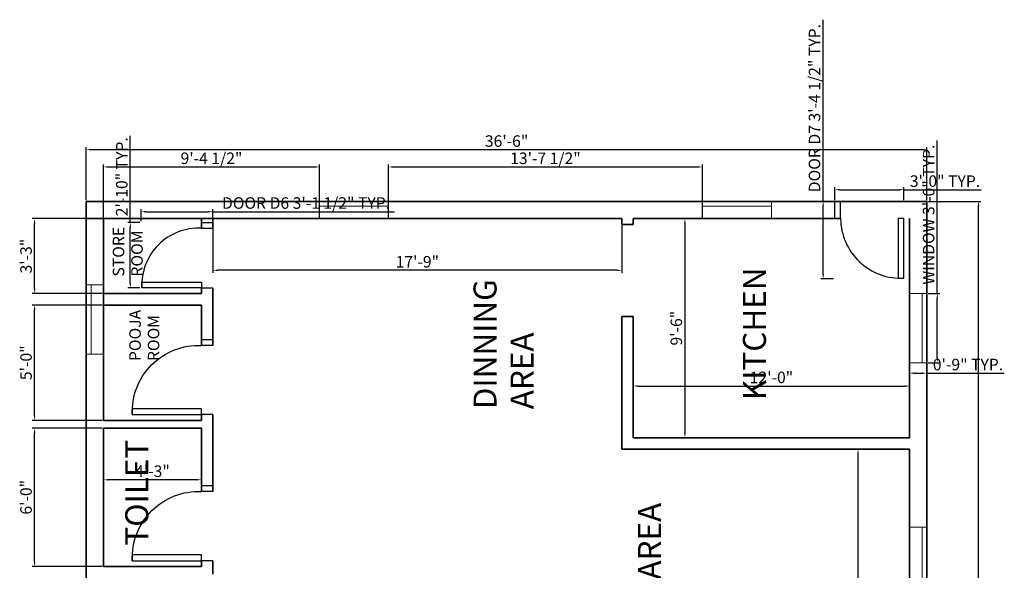
# Model space of a CAD drawing. Units: inches. Extents: x 2641 to 3210, y 2696 to 4064.
# Tile 4 of 4: x 2645 to 3158, y 3777 to 4064. Entities that reach past the tile are written whole.
import ezdxf

# ---------------------------------------------------------------- set-up
doc = ezdxf.new("R2010")
doc.units = ezdxf.units.IN
for name, color, linetype, lineweight in [('A-ANNO-DIMS', 2, 'Continuous', 18), ('A-AREA-IDEN', 7, 'Continuous', 18), ('A-DOOR', 3, 'Continuous', 25), ('A-GLAZ', 4, 'Continuous', 18), ('A-WALL', 7, 'Continuous', 35)]:
    doc.layers.add(name, color=color, linetype=linetype, lineweight=lineweight)
doc.styles.get("Standard").update_dxf_attribs({"font": 'arial.ttf'})
doc.dimstyles.new('ISO-25', dxfattribs={"dimtxt": 6, "dimasz": 2.5, "dimexe": 1.25, "dimexo": 0.625, "dimtad": 1, "dimdec": 1, "dimlunit": 3, "dimtxsty": 'Standard', "dimcen": 2.5, "dimadec": 0, "dimazin": 0, "dimtfac": 1, "dimtdec": 1, "dimtmove": 0, "dimatfit": 3, "dimfxl": 1, "dimarcsym": 0})

# ---------------------------------------------------------------- blocks, each defined once
blk = doc.blocks.new('DOOR-36-INT')
for p, q in [((0, 42.03), (0, 36.03)), ((36, 42.03), (36, 36.03)), ((39, 42.03), (39, 36.03))]:
    blk.add_line(p, q)
blk.add_lwpolyline([(0, 36.03), (3, 36.03), (3, 0.03), (0, 0.03)], close=True)
blk.add_arc((1.5, 34.53), 34.53, 267.5104, 2.4896)
blk = doc.blocks.new('DOOR-31-INT')
for p, q in [((31.04, 34), (37.04, 34)), ((31.04, 31), (37.04, 31)), ((31.04, 0), (37.04, 0))]:
    blk.add_line(p, q)
blk.add_lwpolyline([(31.04, 0), (0.04, 0), (0.04, 3), (31.04, 3)], close=True)
blk.add_arc((29.54, 1.5), 29.54, 87.0892, 182.9108)
blk = doc.blocks.new('DOOR-31-EXT')
for p, q in [((0, 31.04), (0, 40.04)), ((3, 31.04), (3, 40.04))]:
    blk.add_line(p, q)
blk.add_lwpolyline([(36, 31.04), (33, 31.04), (33, 0.04), (36, 0.04)], close=True)
blk.add_arc((34.5, 31.5), 31.5, 180.8507, 272.7291)
blk = doc.blocks.new('WIN-36x9')
blk.add_line((6.5, 36), (6.5, 0))
blk.add_lwpolyline([(9, 36), (0, 36), (0, 0), (9, 0)], close=True)
blk = doc.blocks.new('*D31')
at = {"layer": 'A-ANNO-DIMS', "color": 0, "lineweight": -2, "transparency": 16777216}
for p, q in [((3123.03, 3921.39), (3123.03, 4001.07)), ((3118.25, 3921.39), (3124.28, 3921.39)), ((3123.03, 3887.89), (3123.03, 3918.89)), ((3118.25, 3885.39), (3124.28, 3885.39))]:
    blk.add_line(p, q, dxfattribs=at)
at = {"layer": 'A-ANNO-DIMS', "color": 0, "transparency": 16777216}
for points in [[(3122.61, 3918.89), (3123.44, 3918.89), (3123.03, 3921.39)], [(3122.61, 3887.89), (3123.44, 3887.89), (3123.03, 3885.39)]]:
    blk.add_solid(points, dxfattribs=at)
at = {"layer": 'Defpoints', "color": 0, "transparency": 16777216}
for p in [(3117.63, 3921.39), (3123.03, 3921.39), (3117.63, 3885.39)]:
    blk.add_point(p, dxfattribs=at)
at = {"layer": 'A-ANNO-DIMS', "color": 0, "transparency": 16777216, "insert": (3119.29, 3962.48), "char_height": 6, "attachment_point": 5, "rotation": 90}
blk.add_mtext('WINDOW 3\'-0" TYP.', dxfattribs=at)
blk = doc.blocks.new('*D32')
at = {"layer": 'A-ANNO-DIMS', "color": 0, "lineweight": -2, "transparency": 16777216}
for p, q in [((3108.63, 3884.77), (3108.63, 3878.74)), ((3117.63, 3884.77), (3117.63, 3878.74)), ((3111.13, 3879.99), (3115.13, 3879.99)), ((3117.63, 3879.99), (3157.95, 3879.99))]:
    blk.add_line(p, q, dxfattribs=at)
at = {"layer": 'A-ANNO-DIMS', "color": 0, "transparency": 16777216}
for points in [[(3111.13, 3880.41), (3111.13, 3879.57), (3108.63, 3879.99)], [(3115.13, 3880.41), (3115.13, 3879.57), (3117.63, 3879.99)]]:
    blk.add_solid(points, dxfattribs=at)
at = {"layer": 'Defpoints', "color": 0, "transparency": 16777216}
for p in [(3108.63, 3885.39), (3117.63, 3885.39), (3117.63, 3879.99)]:
    blk.add_point(p, dxfattribs=at)
at = {"layer": 'A-ANNO-DIMS', "color": 0, "transparency": 16777216, "insert": (3139.04, 3883.68), "char_height": 6, "attachment_point": 5}
blk.add_mtext('0\'-9" TYP.', dxfattribs=at)
blk = doc.blocks.new('*D43')
at = {"layer": 'A-ANNO-DIMS', "color": 0, "lineweight": -2, "transparency": 16777216}
for p, q in [((2708.2, 3959.02), (2708.2, 3965.25)), ((2710.7, 3964), (2743.13, 3964)), ((2745.63, 3959.02), (2745.63, 3965.25)), ((2745.63, 3964), (2840.15, 3964))]:
    blk.add_line(p, q, dxfattribs=at)
at = {"layer": 'A-ANNO-DIMS', "color": 0, "transparency": 16777216}
for points in [[(2710.7, 3964.42), (2710.7, 3963.59), (2708.2, 3964)], [(2743.13, 3964.42), (2743.13, 3963.59), (2745.63, 3964)]]:
    blk.add_solid(points, dxfattribs=at)
at = {"layer": 'Defpoints', "color": 0, "transparency": 16777216}
for p in [(2745.63, 3964), (2708.2, 3958.39), (2745.63, 3958.39)]:
    blk.add_point(p, dxfattribs=at)
at = {"layer": 'A-ANNO-DIMS', "color": 0, "transparency": 16777216, "insert": (2794.14, 3967.74), "char_height": 6, "attachment_point": 5}
blk.add_mtext('DOOR D6 3\'-1 1/2" TYP.', dxfattribs=at)
blk = doc.blocks.new('*D44')
at = {"layer": 'A-ANNO-DIMS', "color": 0, "lineweight": -2, "transparency": 16777216}
for p, q in [((2702.59, 3958.39), (2702.59, 4003.48)), ((2707.58, 3958.39), (2701.34, 3958.39)), ((2702.59, 3926.89), (2702.59, 3955.89)), ((2707.58, 3924.39), (2701.34, 3924.39))]:
    blk.add_line(p, q, dxfattribs=at)
at = {"layer": 'A-ANNO-DIMS', "color": 0, "transparency": 16777216}
for points in [[(2702.17, 3955.89), (2703, 3955.89), (2702.59, 3958.39)], [(2702.17, 3926.89), (2703, 3926.89), (2702.59, 3924.39)]]:
    blk.add_solid(points, dxfattribs=at)
at = {"layer": 'Defpoints', "color": 0, "transparency": 16777216}
for p in [(2702.59, 3958.39), (2708.2, 3958.39), (2708.2, 3924.39)]:
    blk.add_point(p, dxfattribs=at)
at = {"layer": 'A-ANNO-DIMS', "color": 0, "transparency": 16777216, "insert": (2698.9, 3982.18), "char_height": 6, "attachment_point": 5, "rotation": 90}
blk.add_mtext('2\'-10" TYP.', dxfattribs=at)
blk = doc.blocks.new('*D45')
at = {"layer": 'A-ANNO-DIMS', "color": 0, "lineweight": -2, "transparency": 16777216}
for p, q in [((3063.56, 3969.39), (3063.56, 4063.91)), ((3069, 3969.39), (3062.31, 3969.39)), ((3063.56, 3931.48), (3063.56, 3966.89)), ((3069, 3928.98), (3062.31, 3928.98))]:
    blk.add_line(p, q, dxfattribs=at)
at = {"layer": 'A-ANNO-DIMS', "color": 0, "transparency": 16777216}
for points in [[(3063.15, 3966.89), (3063.98, 3966.89), (3063.56, 3969.39)], [(3063.15, 3931.48), (3063.98, 3931.48), (3063.56, 3928.98)]]:
    blk.add_solid(points, dxfattribs=at)
at = {"layer": 'Defpoints', "color": 0, "transparency": 16777216}
for p in [(3063.56, 3969.39), (3069.63, 3969.39), (3069.63, 3928.98)]:
    blk.add_point(p, dxfattribs=at)
at = {"layer": 'A-ANNO-DIMS', "color": 0, "transparency": 16777216, "insert": (3059.83, 4017.9), "char_height": 6, "attachment_point": 5, "rotation": 90}
blk.add_mtext('DOOR D7 3\'-4 1/2" TYP.', dxfattribs=at)
blk = doc.blocks.new('*D46')
at = {"layer": 'A-ANNO-DIMS', "color": 0, "lineweight": -2, "transparency": 16777216}
for p, q in [((3069.63, 3970.02), (3069.63, 3976.7)), ((3105.63, 3970.02), (3105.63, 3976.7)), ((3072.13, 3975.45), (3103.13, 3975.45)), ((3105.63, 3975.45), (3145.94, 3975.45))]:
    blk.add_line(p, q, dxfattribs=at)
at = {"layer": 'A-ANNO-DIMS', "color": 0, "transparency": 16777216}
for points in [[(3072.13, 3975.87), (3072.13, 3975.03), (3069.63, 3975.45)], [(3103.13, 3975.87), (3103.13, 3975.03), (3105.63, 3975.45)]]:
    blk.add_solid(points, dxfattribs=at)
at = {"layer": 'Defpoints', "color": 0, "transparency": 16777216}
for p in [(3105.63, 3975.45), (3069.63, 3969.39), (3105.63, 3969.39)]:
    blk.add_point(p, dxfattribs=at)
at = {"layer": 'A-ANNO-DIMS', "color": 0, "transparency": 16777216, "insert": (3127.04, 3979.14), "char_height": 6, "attachment_point": 5}
blk.add_mtext('3\'-0" TYP.', dxfattribs=at)
blk = doc.blocks.new('*D66')
at = {"layer": 'A-ANNO-DIMS', "color": 0, "lineweight": -2, "transparency": 16777216}
for p, q in [((2679.63, 3970.02), (2679.63, 3997.54)), ((2682.13, 3996.29), (3115.13, 3996.29)), ((3117.63, 3970.02), (3117.63, 3997.54))]:
    blk.add_line(p, q, dxfattribs=at)
at = {"layer": 'A-ANNO-DIMS', "color": 0, "transparency": 16777216}
for points in [[(2682.13, 3996.71), (2682.13, 3995.87), (2679.63, 3996.29)], [(3115.13, 3996.71), (3115.13, 3995.87), (3117.63, 3996.29)]]:
    blk.add_solid(points, dxfattribs=at)
at = {"layer": 'Defpoints', "color": 0, "transparency": 16777216}
for p in [(3117.63, 3996.29), (2679.63, 3969.39), (3117.63, 3969.39)]:
    blk.add_point(p, dxfattribs=at)
at = {"layer": 'A-ANNO-DIMS', "color": 0, "transparency": 16777216, "insert": (2898.63, 3999.98), "char_height": 6, "attachment_point": 5}
blk.add_mtext('36\'-6"', dxfattribs=at)
blk = doc.blocks.new('*D67')
at = {"layer": 'A-ANNO-DIMS', "color": 0, "lineweight": -2, "transparency": 16777216}
for p, q in [((3118.25, 3969.39), (3145.78, 3969.39)), ((3144.53, 3455.89), (3144.53, 3966.89)), ((3073.25, 3453.39), (3145.78, 3453.39))]:
    blk.add_line(p, q, dxfattribs=at)
at = {"layer": 'A-ANNO-DIMS', "color": 0, "transparency": 16777216}
for points in [[(3144.11, 3966.89), (3144.94, 3966.89), (3144.53, 3969.39)], [(3144.11, 3455.89), (3144.94, 3455.89), (3144.53, 3453.39)]]:
    blk.add_solid(points, dxfattribs=at)
at = {"layer": 'Defpoints', "color": 0, "transparency": 16777216}
for p in [(3117.63, 3969.39), (3144.53, 3969.39), (3072.63, 3453.39)]:
    blk.add_point(p, dxfattribs=at)
at = {"layer": 'A-ANNO-DIMS', "color": 0, "transparency": 16777216, "insert": (3140.84, 3711.39), "char_height": 6, "attachment_point": 5, "rotation": 90}
blk.add_mtext('43\'-0"', dxfattribs=at)
blk = doc.blocks.new('*D72')
at = {"layer": 'A-ANNO-DIMS', "color": 0, "lineweight": -2, "transparency": 16777216}
for p, q in [((2688, 3851.39), (2651.48, 3851.39)), ((2652.73, 3781.89), (2652.73, 3848.89)), ((2688, 3779.39), (2651.48, 3779.39))]:
    blk.add_line(p, q, dxfattribs=at)
at = {"layer": 'A-ANNO-DIMS', "color": 0, "transparency": 16777216}
for points in [[(2652.31, 3848.89), (2653.14, 3848.89), (2652.73, 3851.39)], [(2652.31, 3781.89), (2653.14, 3781.89), (2652.73, 3779.39)]]:
    blk.add_solid(points, dxfattribs=at)
at = {"layer": 'Defpoints', "color": 0, "transparency": 16777216}
for p in [(2652.73, 3851.39), (2688.63, 3851.39), (2688.63, 3779.39)]:
    blk.add_point(p, dxfattribs=at)
at = {"layer": 'A-ANNO-DIMS', "color": 0, "transparency": 16777216, "insert": (2649.04, 3815.39), "char_height": 6, "attachment_point": 5, "rotation": 90}
blk.add_mtext('6\'-0"', dxfattribs=at)
blk = doc.blocks.new('*D73')
at = {"layer": 'A-ANNO-DIMS', "color": 0, "lineweight": -2, "transparency": 16777216}
for p, q in [((2688, 3915.39), (2651.48, 3915.39)), ((2652.73, 3857.89), (2652.73, 3912.89)), ((2688, 3855.39), (2651.48, 3855.39))]:
    blk.add_line(p, q, dxfattribs=at)
at = {"layer": 'A-ANNO-DIMS', "color": 0, "transparency": 16777216}
for points in [[(2652.31, 3912.89), (2653.14, 3912.89), (2652.73, 3915.39)], [(2652.31, 3857.89), (2653.14, 3857.89), (2652.73, 3855.39)]]:
    blk.add_solid(points, dxfattribs=at)
at = {"layer": 'Defpoints', "color": 0, "transparency": 16777216}
for p in [(2652.73, 3915.39), (2688.63, 3915.39), (2688.63, 3855.39)]:
    blk.add_point(p, dxfattribs=at)
at = {"layer": 'A-ANNO-DIMS', "color": 0, "transparency": 16777216, "insert": (2649.04, 3885.39), "char_height": 6, "attachment_point": 5, "rotation": 90}
blk.add_mtext('5\'-0"', dxfattribs=at)
blk = doc.blocks.new('*D74')
at = {"layer": 'A-ANNO-DIMS', "color": 0, "lineweight": -2, "transparency": 16777216}
for p, q in [((2688, 3960.39), (2651.48, 3960.39)), ((2652.73, 3923.89), (2652.73, 3957.89)), ((2688, 3921.39), (2651.48, 3921.39))]:
    blk.add_line(p, q, dxfattribs=at)
at = {"layer": 'A-ANNO-DIMS', "color": 0, "transparency": 16777216}
for points in [[(2652.31, 3957.89), (2653.14, 3957.89), (2652.73, 3960.39)], [(2652.31, 3923.89), (2653.14, 3923.89), (2652.73, 3921.39)]]:
    blk.add_solid(points, dxfattribs=at)
at = {"layer": 'Defpoints', "color": 0, "transparency": 16777216}
for p in [(2652.73, 3960.39), (2688.63, 3960.39), (2688.63, 3921.39)]:
    blk.add_point(p, dxfattribs=at)
at = {"layer": 'A-ANNO-DIMS', "color": 0, "transparency": 16777216, "insert": (2649.04, 3940.89), "char_height": 6, "attachment_point": 5, "rotation": 90}
blk.add_mtext('3\'-3"', dxfattribs=at)
blk = doc.blocks.new('*D75')
at = {"layer": 'A-ANNO-DIMS', "color": 0, "lineweight": -2, "transparency": 16777216}
for p, q in [((2688.63, 3850.77), (2688.63, 3823.24)), ((2739.63, 3850.77), (2739.63, 3823.24)), ((2737.13, 3824.49), (2691.13, 3824.49))]:
    blk.add_line(p, q, dxfattribs=at)
at = {"layer": 'A-ANNO-DIMS', "color": 0, "transparency": 16777216}
for points in [[(2691.13, 3824.91), (2691.13, 3824.07), (2688.63, 3824.49)], [(2737.13, 3824.91), (2737.13, 3824.07), (2739.63, 3824.49)]]:
    blk.add_solid(points, dxfattribs=at)
at = {"layer": 'Defpoints', "color": 0, "transparency": 16777216}
for p in [(2688.63, 3851.39), (2739.63, 3851.39), (2688.63, 3824.49)]:
    blk.add_point(p, dxfattribs=at)
at = {"layer": 'A-ANNO-DIMS', "color": 0, "transparency": 16777216, "insert": (2714.13, 3828.18), "char_height": 6, "attachment_point": 5}
blk.add_mtext('4\'-3"', dxfattribs=at)
blk = doc.blocks.new('*D76')
at = {"layer": 'A-ANNO-DIMS', "color": 0, "lineweight": -2, "transparency": 16777216}
for p, q in [((2964.63, 3847.02), (2964.63, 3874.54)), ((2967.13, 3873.29), (3106.13, 3873.29)), ((3108.63, 3847.02), (3108.63, 3874.54))]:
    blk.add_line(p, q, dxfattribs=at)
at = {"layer": 'A-ANNO-DIMS', "color": 0, "transparency": 16777216}
for points in [[(2967.13, 3873.71), (2967.13, 3872.87), (2964.63, 3873.29)], [(3106.13, 3873.71), (3106.13, 3872.87), (3108.63, 3873.29)]]:
    blk.add_solid(points, dxfattribs=at)
at = {"layer": 'Defpoints', "color": 0, "transparency": 16777216}
for p in [(3108.63, 3873.29), (2964.63, 3846.39), (3108.63, 3846.39)]:
    blk.add_point(p, dxfattribs=at)
at = {"layer": 'A-ANNO-DIMS', "color": 0, "transparency": 16777216, "insert": (3036.63, 3876.98), "char_height": 6, "attachment_point": 5}
blk.add_mtext('12\'-0"', dxfattribs=at)
blk = doc.blocks.new('*D77')
at = {"layer": 'A-ANNO-DIMS', "color": 0, "lineweight": -2, "transparency": 16777216}
for p, q in [((2965.25, 3960.39), (2992.78, 3960.39)), ((2991.53, 3957.89), (2991.53, 3848.89)), ((2965.25, 3846.39), (2992.78, 3846.39))]:
    blk.add_line(p, q, dxfattribs=at)
at = {"layer": 'A-ANNO-DIMS', "color": 0, "transparency": 16777216}
for points in [[(2991.11, 3957.89), (2991.94, 3957.89), (2991.53, 3960.39)], [(2991.11, 3848.89), (2991.94, 3848.89), (2991.53, 3846.39)]]:
    blk.add_solid(points, dxfattribs=at)
at = {"layer": 'Defpoints', "color": 0, "transparency": 16777216}
for p in [(2964.63, 3960.39), (2964.63, 3846.39), (2991.53, 3846.39)]:
    blk.add_point(p, dxfattribs=at)
at = {"layer": 'A-ANNO-DIMS', "color": 0, "transparency": 16777216, "insert": (2987.84, 3903.39), "char_height": 6, "attachment_point": 5, "rotation": 90}
blk.add_mtext('9\'-6"', dxfattribs=at)
blk = doc.blocks.new('*D78')
at = {"layer": 'A-ANNO-DIMS', "color": 0, "lineweight": -2, "transparency": 16777216}
for p, q in [((2745.63, 3959.77), (2745.63, 3932.24)), ((2958.63, 3959.77), (2958.63, 3932.24)), ((2956.13, 3933.49), (2748.13, 3933.49))]:
    blk.add_line(p, q, dxfattribs=at)
at = {"layer": 'A-ANNO-DIMS', "color": 0, "transparency": 16777216}
for points in [[(2748.13, 3933.91), (2748.13, 3933.07), (2745.63, 3933.49)], [(2956.13, 3933.91), (2956.13, 3933.07), (2958.63, 3933.49)]]:
    blk.add_solid(points, dxfattribs=at)
at = {"layer": 'Defpoints', "color": 0, "transparency": 16777216}
for p in [(2745.63, 3960.39), (2958.63, 3960.39), (2745.63, 3933.49)]:
    blk.add_point(p, dxfattribs=at)
at = {"layer": 'A-ANNO-DIMS', "color": 0, "transparency": 16777216, "insert": (2852.13, 3937.18), "char_height": 6, "attachment_point": 5}
blk.add_mtext('17\'-9"', dxfattribs=at)
blk = doc.blocks.new('*D80')
at = {"layer": 'A-ANNO-DIMS', "color": 0, "lineweight": -2, "transparency": 16777216}
for p, q in [((3108, 3840.39), (3080.48, 3840.39)), ((3081.73, 3662.89), (3081.73, 3837.89)), ((3108, 3660.39), (3080.48, 3660.39))]:
    blk.add_line(p, q, dxfattribs=at)
at = {"layer": 'A-ANNO-DIMS', "color": 0, "transparency": 16777216}
for points in [[(3081.31, 3837.89), (3082.14, 3837.89), (3081.73, 3840.39)], [(3081.31, 3662.89), (3082.14, 3662.89), (3081.73, 3660.39)]]:
    blk.add_solid(points, dxfattribs=at)
at = {"layer": 'Defpoints', "color": 0, "transparency": 16777216}
for p in [(3081.73, 3840.39), (3108.63, 3840.39), (3108.63, 3660.39)]:
    blk.add_point(p, dxfattribs=at)
at = {"layer": 'A-ANNO-DIMS', "color": 0, "transparency": 16777216, "insert": (3078.04, 3750.39), "char_height": 6, "attachment_point": 5, "rotation": 90}
blk.add_mtext('15\'-0"', dxfattribs=at)
blk = doc.blocks.new('*D81')
at = {"layer": 'A-ANNO-DIMS', "color": 0, "lineweight": -2, "transparency": 16777216}
for p, q in [((2688.63, 3961.02), (2688.63, 3988.54)), ((2691.13, 3987.29), (2798.63, 3987.29)), ((2801.13, 3961.02), (2801.13, 3988.54))]:
    blk.add_line(p, q, dxfattribs=at)
at = {"layer": 'A-ANNO-DIMS', "color": 0, "transparency": 16777216}
for points in [[(2691.13, 3987.71), (2691.13, 3986.87), (2688.63, 3987.29)], [(2798.63, 3987.71), (2798.63, 3986.87), (2801.13, 3987.29)]]:
    blk.add_solid(points, dxfattribs=at)
at = {"layer": 'Defpoints', "color": 0, "transparency": 16777216}
for p in [(2801.13, 3987.29), (2688.63, 3960.39), (2801.13, 3960.39)]:
    blk.add_point(p, dxfattribs=at)
at = {"layer": 'A-ANNO-DIMS', "color": 0, "transparency": 16777216, "insert": (2744.88, 3991.02), "char_height": 6, "attachment_point": 5}
blk.add_mtext('9\'-4 1/2"', dxfattribs=at)
blk = doc.blocks.new('*D82')
at = {"layer": 'A-ANNO-DIMS', "color": 0, "lineweight": -2, "transparency": 16777216}
for p, q in [((2837.13, 3961.02), (2837.13, 3988.54)), ((2839.63, 3987.29), (2998.13, 3987.29)), ((3000.63, 3961.02), (3000.63, 3988.54))]:
    blk.add_line(p, q, dxfattribs=at)
at = {"layer": 'A-ANNO-DIMS', "color": 0, "transparency": 16777216}
for points in [[(2839.63, 3987.71), (2839.63, 3986.87), (2837.13, 3987.29)], [(2998.13, 3987.71), (2998.13, 3986.87), (3000.63, 3987.29)]]:
    blk.add_solid(points, dxfattribs=at)
at = {"layer": 'Defpoints', "color": 0, "transparency": 16777216}
for p in [(3000.63, 3987.29), (2837.13, 3960.39), (3000.63, 3960.39)]:
    blk.add_point(p, dxfattribs=at)
at = {"layer": 'A-ANNO-DIMS', "color": 0, "transparency": 16777216, "insert": (2918.88, 3991.02), "char_height": 6, "attachment_point": 5}
blk.add_mtext('13\'-7 1/2"', dxfattribs=at)

msp = doc.modelspace()

# ---------------------------------------------------------------- linework, layer by layer
at = {"layer": 'A-WALL'}
for p, q in [((2679.63, 3453.39), (2679.63, 3969.39)), ((2679.63, 3960.39), (2958.63, 3960.39)), ((2688.63, 3855.39), (2688.63, 3960.39)), ((2739.63, 3955.39), (2739.63, 3960.39)), ((2745.63, 3955.39), (2745.63, 3960.39)), ((2958.63, 3960.39), (2958.63, 3957.39)), ((2958.63, 3960.39), (2958.63, 3957.39)), ((2964.63, 3960.39), (3072.63, 3960.39)), ((2964.63, 3960.39), (2964.63, 3957.39)), ((3108.63, 3960.39), (3108.63, 3846.39)), ((2958.63, 3957.39), (2964.63, 3957.39)), ((2688.63, 3921.39), (2739.63, 3921.39)), ((2739.63, 3921.39), (2739.63, 3924.39)), ((2739.63, 3921.39), (2739.63, 3924.39)), ((2745.63, 3894.39), (2745.63, 3924.39)), ((2688.63, 3915.39), (2739.63, 3915.39)), ((2739.63, 3894.39), (2739.63, 3915.39)), ((2958.63, 3909.39), (2958.63, 3840.39)), ((2958.63, 3909.39), (2964.63, 3909.39)), ((2964.63, 3909.39), (2964.63, 3846.39)), ((2739.63, 3855.39), (2739.63, 3858.39)), ((2739.63, 3855.39), (2739.63, 3858.39)), ((2745.63, 3818.39), (2745.63, 3858.39)), ((2688.63, 3855.39), (2739.63, 3855.39)), ((2688.63, 3779.39), (2688.63, 3851.39)), ((2688.63, 3851.39), (2739.63, 3851.39)), ((2739.63, 3818.39), (2739.63, 3851.39)), ((3108.63, 3846.39), (2964.63, 3846.39)), ((3108.63, 3840.39), (2958.63, 3840.39)), ((3108.63, 3840.39), (3108.63, 3723.39)), ((2739.63, 3779.39), (2739.63, 3782.39)), ((2739.63, 3779.39), (2739.63, 3782.39)), ((2745.63, 3775.39), (2745.63, 3782.39)), ((2688.63, 3779.39), (2739.63, 3779.39))]:
    msp.add_line(p, q, dxfattribs=at)
for points in [[(2679.63, 3969.39), (3072.63, 3969.39)], [(3072.63, 3969.39), (3117.63, 3969.39), (3117.63, 3723.39)]]:
    msp.add_lwpolyline(points, dxfattribs=at)

# ---------------------------------------------------------------- block references
at = {"layer": 'A-DOOR'}
for name, p in [('DOOR-31-EXT', (3069.63, 3929.35)), ('DOOR-31-INT', (2708.59, 3924.39))]:
    msp.add_blockref(name, p, dxfattribs=at)
at = {"layer": 'A-DOOR', "extrusion": (0, 0, -1), "zscale": -1, "rotation": 89.99999999999683}
for p in [(-2703.59, 3858.39), (-2703.59, 3782.39)]:
    msp.add_blockref('DOOR-36-INT', p, dxfattribs=at)
at = {"layer": 'A-GLAZ'}
for p, rotation in [((2837.13, 3960.39), 90.00000000000236), ((3036.63, 3960.39), 90.00000000000063), ((2688.63, 3925.89), 180)]:
    msp.add_blockref('WIN-36x9', p, dxfattribs=dict(at, rotation=rotation))
for p in [(3108.63, 3885.39), (3108.63, 3763.89)]:
    msp.add_blockref('WIN-36x9', p, dxfattribs=at)

# ---------------------------------------------------------------- texts
at = {"layer": 'A-AREA-IDEN'}
for s, height, p in [('STORE', 6, (2699.44, 3930.24)), ('ROOM', 6, (2709.08, 3930.24)), ('KITCHEN', 12, (3033.77, 3865.95)), ('DINNING', 12, (2893.39, 3861.21)), ('POOJA', 6, (2708.06, 3886.26)), ('ROOM', 6, (2717.7, 3886.26)), ('AREA', 12, (2912.67, 3861.21)), ('TOILET', 12, (2711.95, 3790.22)), ('HALL/LIVING AREA', 12, (2979.08, 3671.82))]:
    msp.add_text(s, height=height, rotation=90, dxfattribs=at).set_placement(p)

# ---------------------------------------------------------------- dimensions: what is measured, and where the dimension line sits
at = {"layer": 'A-ANNO-DIMS'}
for base, p1, p2, text, picture, middle in [((3063.56, 3969.39), (3069.63, 3928.98), (3069.63, 3969.39), 'DOOR D7 <> TYP.', '*D45', (3059.83, 4017.9)), ((2702.59, 3958.39), (2708.2, 3924.39), (2708.2, 3958.39), '<> TYP.', '*D44', (2698.9, 3982.18)), ((3123.03, 3921.39), (3117.63, 3885.39), (3117.63, 3921.39), 'WINDOW <> TYP.', '*D31', (3119.29, 3962.48))]:
    dim = msp.add_linear_dim(base=base, p1=p1, p2=p2, angle=90, text=text, dimstyle='ISO-25', override={"dimdec": 1, "dimlfac": 1, "dimrnd": 0, "dimzin": 1, "dimdsep": 46, "dimlunit": 4, "dimfrac": 2}, dxfattribs=at)
    dim.commit()
    dim.dimension.update_dxf_attribs({"geometry": picture, "text_midpoint": middle})
for base, p1, p2, picture, middle in [((3117.63, 3996.29), (2679.63, 3969.39), (3117.63, 3969.39), '*D66', (2898.63, 3999.98)), ((2801.13, 3987.29), (2688.63, 3960.39), (2801.13, 3960.39), '*D81', (2744.88, 3991.02)), ((3000.63, 3987.29), (2837.13, 3960.39), (3000.63, 3960.39), '*D82', (2918.88, 3991.02)), ((3108.63, 3873.29), (2964.63, 3846.39), (3108.63, 3846.39), '*D76', (3036.63, 3876.98))]:
    dim = msp.add_linear_dim(base=base, p1=p1, p2=p2, dimstyle='ISO-25', override={"dimdec": 1, "dimlfac": 1, "dimrnd": 0, "dimzin": 1, "dimdsep": 46, "dimlunit": 4, "dimfrac": 2}, dxfattribs=at)
    dim.commit()
    dim.dimension.update_dxf_attribs({"geometry": picture, "text_midpoint": middle})
for base, p1, p2, text, picture, middle in [((2745.63, 3964), (2708.2, 3958.39), (2745.63, 3958.39), 'DOOR D6 <> TYP.', '*D43', (2794.14, 3967.74)), ((3105.63, 3975.45), (3069.63, 3969.39), (3105.63, 3969.39), '<> TYP.', '*D46', (3127.04, 3979.14)), ((3117.63, 3879.99), (3108.63, 3885.39), (3117.63, 3885.39), '<> TYP.', '*D32', (3139.04, 3883.68))]:
    dim = msp.add_linear_dim(base=base, p1=p1, p2=p2, text=text, dimstyle='ISO-25', override={"dimdec": 1, "dimlfac": 1, "dimrnd": 0, "dimzin": 1, "dimdsep": 46, "dimlunit": 4, "dimfrac": 2}, dxfattribs=at)
    dim.commit()
    dim.dimension.update_dxf_attribs({"geometry": picture, "text_midpoint": middle})
for base, p1, p2, angle, picture, middle in [((3144.53, 3969.39), (3072.63, 3453.39), (3117.63, 3969.39), 90, '*D67', (3140.84, 3711.39)), ((2652.73, 3960.39), (2688.63, 3921.39), (2688.63, 3960.39), 90, '*D74', (2649.04, 3940.89)), ((2745.63, 3933.49), (2958.63, 3960.39), (2745.63, 3960.39), 180, '*D78', (2852.13, 3937.18)), ((2991.53, 3846.39), (2964.63, 3960.39), (2964.63, 3846.39), 270, '*D77', (2987.84, 3903.39)), ((2652.73, 3915.39), (2688.63, 3855.39), (2688.63, 3915.39), 90, '*D73', (2649.04, 3885.39)), ((2652.73, 3851.39), (2688.63, 3779.39), (2688.63, 3851.39), 90, '*D72', (2649.04, 3815.39)), ((2688.63, 3824.49), (2739.63, 3851.39), (2688.63, 3851.39), 180, '*D75', (2714.13, 3828.18)), ((3081.73, 3840.39), (3108.63, 3660.39), (3108.63, 3840.39), 90, '*D80', (3078.04, 3750.39))]:
    dim = msp.add_linear_dim(base=base, p1=p1, p2=p2, angle=angle, dimstyle='ISO-25', override={"dimdec": 1, "dimlfac": 1, "dimrnd": 0, "dimzin": 1, "dimdsep": 46, "dimlunit": 4, "dimfrac": 2}, dxfattribs=at)
    dim.commit()
    dim.dimension.update_dxf_attribs({"geometry": picture, "text_midpoint": middle})

doc.saveas('drawing.dxf')
